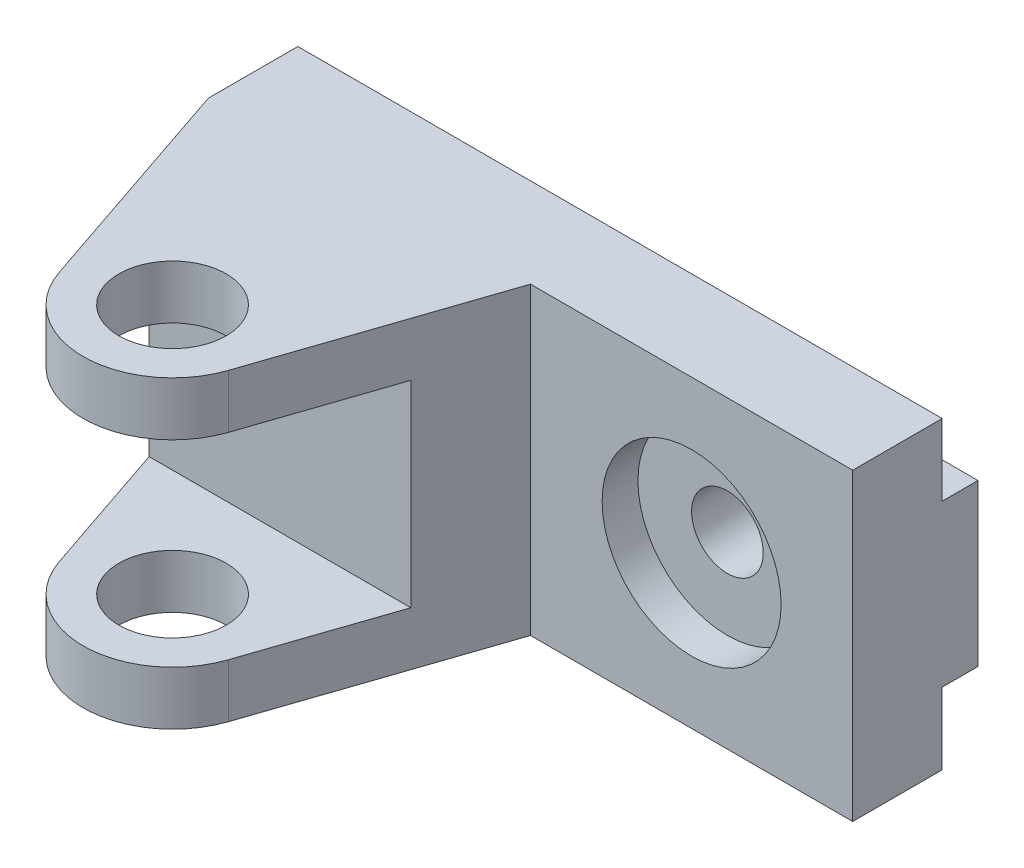
ISO-10303-21;
HEADER;
FILE_DESCRIPTION(('STEP AP214'),'2;1');
FILE_NAME('part.step','',(''),(''),'','','');
FILE_SCHEMA(('AUTOMOTIVE_DESIGN { 1 0 10303 214 1 1 1 1 }'));
ENDSEC;
DATA;
#1=APPLICATION_CONTEXT('core data for automotive mechanical design processes');
#2=APPLICATION_PROTOCOL_DEFINITION('international standard','automotive_design',2000,#1);
#3=PRODUCT_CONTEXT('',#1,'mechanical');
#4=PRODUCT('Part','Part','',(#3));
#5=PRODUCT_RELATED_PRODUCT_CATEGORY('part','',(#4));
#6=PRODUCT_DEFINITION_FORMATION('','',#4);
#7=PRODUCT_DEFINITION_CONTEXT('part definition',#1,'design');
#8=PRODUCT_DEFINITION('design','',#6,#7);
#9=PRODUCT_DEFINITION_SHAPE('','',#8);
#10=(LENGTH_UNIT() NAMED_UNIT(*) SI_UNIT(.MILLI.,.METRE.));
#11=(NAMED_UNIT(*) PLANE_ANGLE_UNIT() SI_UNIT($,.RADIAN.));
#12=(NAMED_UNIT(*) SI_UNIT($,.STERADIAN.) SOLID_ANGLE_UNIT());
#13=UNCERTAINTY_MEASURE_WITH_UNIT(LENGTH_MEASURE(1.E-05),#10,'distance_accuracy_value','');
#14=(GEOMETRIC_REPRESENTATION_CONTEXT(3) GLOBAL_UNCERTAINTY_ASSIGNED_CONTEXT((#13)) GLOBAL_UNIT_ASSIGNED_CONTEXT((#10,
#11,#12)) REPRESENTATION_CONTEXT('',''));
#15=CARTESIAN_POINT('',(0.,0.,0.));
#16=DIRECTION('',(0.,0.,1.));
#17=DIRECTION('',(1.,0.,0.));
#18=AXIS2_PLACEMENT_3D('',#15,#16,#17);
#19=CARTESIAN_POINT('',(0.,0.,25.));
#20=DIRECTION('',(0.,0.,-1.));
#21=DIRECTION('',(-1.,0.,0.));
#22=AXIS2_PLACEMENT_3D('',#19,#20,#21);
#23=PLANE('',#22);
#24=CARTESIAN_POINT('',(45.,0.,25.));
#25=DIRECTION('',(0.,0.,1.));
#26=DIRECTION('',(1.,0.,0.));
#27=AXIS2_PLACEMENT_3D('',#24,#25,#26);
#28=CIRCLE('',#27,25.);
#29=CARTESIAN_POINT('',(70.,0.,25.));
#30=VERTEX_POINT('',#29);
#31=EDGE_CURVE('E242',#30,#30,#28,.T.);
#32=ORIENTED_EDGE('',*,*,#31,.F.);
#33=EDGE_LOOP('',(#32));
#34=FACE_BOUND('',#33,.T.);
#35=DIRECTION('',(-1.,0.,0.));
#36=VECTOR('',#35,1.);
#37=CARTESIAN_POINT('',(-90.,42.5,25.));
#38=LINE('',#37,#36);
#39=CARTESIAN_POINT('',(90.,42.5,25.));
#40=VERTEX_POINT('',#39);
#41=CARTESIAN_POINT('',(0.,42.5,25.));
#42=VERTEX_POINT('',#41);
#43=EDGE_CURVE('E251',#40,#42,#38,.T.);
#44=ORIENTED_EDGE('',*,*,#43,.T.);
#45=DIRECTION('',(0.,-1.,0.));
#46=VECTOR('',#45,1.);
#47=CARTESIAN_POINT('',(0.,-27.5,25.));
#48=LINE('',#47,#46);
#49=CARTESIAN_POINT('',(0.,-42.5,25.));
#50=VERTEX_POINT('',#49);
#51=EDGE_CURVE('E62',#42,#50,#48,.T.);
#52=ORIENTED_EDGE('',*,*,#51,.T.);
#53=DIRECTION('',(1.,0.,0.));
#54=VECTOR('',#53,1.);
#55=CARTESIAN_POINT('',(-90.,-42.5,25.));
#56=LINE('',#55,#54);
#57=CARTESIAN_POINT('',(90.,-42.5,25.));
#58=VERTEX_POINT('',#57);
#59=EDGE_CURVE('E256',#50,#58,#56,.T.);
#60=ORIENTED_EDGE('',*,*,#59,.T.);
#61=DIRECTION('',(0.,1.,0.));
#62=VECTOR('',#61,1.);
#63=CARTESIAN_POINT('',(90.,-42.5,25.));
#64=LINE('',#63,#62);
#65=EDGE_CURVE('E252',#58,#40,#64,.T.);
#66=ORIENTED_EDGE('',*,*,#65,.T.);
#67=EDGE_LOOP('',(#44,#52,#60,#66));
#68=FACE_BOUND('',#67,.T.);
#69=ADVANCED_FACE('F39',(#34,#68),#23,.F.);
#70=CARTESIAN_POINT('',(0.,0.,0.));
#71=DIRECTION('',(0.,0.,-1.));
#72=DIRECTION('',(-1.,0.,0.));
#73=AXIS2_PLACEMENT_3D('',#70,#71,#72);
#74=PLANE('',#73);
#75=DIRECTION('',(0.,1.,0.));
#76=VECTOR('',#75,1.);
#77=CARTESIAN_POINT('',(90.,-42.5,0.));
#78=LINE('',#77,#76);
#79=CARTESIAN_POINT('',(90.,22.5,0.));
#80=VERTEX_POINT('',#79);
#81=CARTESIAN_POINT('',(90.,42.5,0.));
#82=VERTEX_POINT('',#81);
#83=EDGE_CURVE('E247',#80,#82,#78,.T.);
#84=ORIENTED_EDGE('',*,*,#83,.F.);
#85=DIRECTION('',(-1.,0.,0.));
#86=VECTOR('',#85,1.);
#87=CARTESIAN_POINT('',(90.,22.5,0.));
#88=LINE('',#87,#86);
#89=CARTESIAN_POINT('',(-90.,22.5,0.));
#90=VERTEX_POINT('',#89);
#91=EDGE_CURVE('E221',#80,#90,#88,.T.);
#92=ORIENTED_EDGE('',*,*,#91,.T.);
#93=DIRECTION('',(0.,-1.,0.));
#94=VECTOR('',#93,1.);
#95=CARTESIAN_POINT('',(-90.,-42.5,0.));
#96=LINE('',#95,#94);
#97=CARTESIAN_POINT('',(-90.,42.5,0.));
#98=VERTEX_POINT('',#97);
#99=EDGE_CURVE('E267',#98,#90,#96,.T.);
#100=ORIENTED_EDGE('',*,*,#99,.F.);
#101=DIRECTION('',(-1.,0.,0.));
#102=VECTOR('',#101,1.);
#103=CARTESIAN_POINT('',(-90.,42.5,0.));
#104=LINE('',#103,#102);
#105=EDGE_CURVE('E263',#82,#98,#104,.T.);
#106=ORIENTED_EDGE('',*,*,#105,.F.);
#107=EDGE_LOOP('',(#84,#92,#100,#106));
#108=FACE_BOUND('',#107,.T.);
#109=ADVANCED_FACE('F316',(#108),#74,.T.);
#110=CARTESIAN_POINT('',(90.,-42.5,25.));
#111=DIRECTION('',(-1.,0.,0.));
#112=DIRECTION('',(0.,0.,1.));
#113=AXIS2_PLACEMENT_3D('',#110,#111,#112);
#114=PLANE('',#113);
#115=CARTESIAN_POINT('',(90.,-42.5,0.));
#116=VERTEX_POINT('',#115);
#117=CARTESIAN_POINT('',(90.,-22.5,0.));
#118=VERTEX_POINT('',#117);
#119=EDGE_CURVE('E264',#116,#118,#78,.T.);
#120=ORIENTED_EDGE('',*,*,#119,.T.);
#121=DIRECTION('',(0.,0.,1.));
#122=VECTOR('',#121,1.);
#123=CARTESIAN_POINT('',(90.,-22.5,0.));
#124=LINE('',#123,#122);
#125=CARTESIAN_POINT('',(90.,-22.5,-9.99999999999999));
#126=VERTEX_POINT('',#125);
#127=EDGE_CURVE('E222',#126,#118,#124,.T.);
#128=ORIENTED_EDGE('',*,*,#127,.F.);
#129=DIRECTION('',(0.,-1.,0.));
#130=VECTOR('',#129,1.);
#131=CARTESIAN_POINT('',(90.,22.5,-9.99999999999999));
#132=LINE('',#131,#130);
#133=CARTESIAN_POINT('',(90.,22.5,-9.99999999999999));
#134=VERTEX_POINT('',#133);
#135=EDGE_CURVE('E216',#134,#126,#132,.T.);
#136=ORIENTED_EDGE('',*,*,#135,.F.);
#137=DIRECTION('',(0.,0.,-1.));
#138=VECTOR('',#137,1.);
#139=CARTESIAN_POINT('',(90.,22.5,0.));
#140=LINE('',#139,#138);
#141=EDGE_CURVE('E217',#80,#134,#140,.T.);
#142=ORIENTED_EDGE('',*,*,#141,.F.);
#143=ORIENTED_EDGE('',*,*,#83,.T.);
#144=DIRECTION('',(0.,0.,-1.));
#145=VECTOR('',#144,1.);
#146=CARTESIAN_POINT('',(90.,42.5,25.));
#147=LINE('',#146,#145);
#148=EDGE_CURVE('E160',#40,#82,#147,.T.);
#149=ORIENTED_EDGE('',*,*,#148,.F.);
#150=ORIENTED_EDGE('',*,*,#65,.F.);
#151=DIRECTION('',(0.,0.,-1.));
#152=VECTOR('',#151,1.);
#153=CARTESIAN_POINT('',(90.,-42.5,25.));
#154=LINE('',#153,#152);
#155=EDGE_CURVE('E262',#58,#116,#154,.T.);
#156=ORIENTED_EDGE('',*,*,#155,.T.);
#157=EDGE_LOOP('',(#120,#128,#136,#142,#143,#149,#150,#156));
#158=FACE_BOUND('',#157,.T.);
#159=ADVANCED_FACE('F41',(#158),#114,.F.);
#160=CARTESIAN_POINT('',(-90.,42.5,25.));
#161=DIRECTION('',(0.,-1.,0.));
#162=DIRECTION('',(0.,0.,-1.));
#163=AXIS2_PLACEMENT_3D('',#160,#161,#162);
#164=PLANE('',#163);
#165=ORIENTED_EDGE('',*,*,#105,.T.);
#166=DIRECTION('',(0.,0.,-1.));
#167=VECTOR('',#166,1.);
#168=CARTESIAN_POINT('',(-90.,42.5,25.));
#169=LINE('',#168,#167);
#170=CARTESIAN_POINT('',(-90.,42.5,25.));
#171=VERTEX_POINT('',#170);
#172=EDGE_CURVE('E280',#171,#98,#169,.T.);
#173=ORIENTED_EDGE('',*,*,#172,.F.);
#174=DIRECTION('',(0.320481248816092,0.,0.947254859664113));
#175=VECTOR('',#174,1.);
#176=CARTESIAN_POINT('',(-90.,42.5,25.));
#177=LINE('',#176,#175);
#178=CARTESIAN_POINT('',(-68.6813714916028,42.5,88.0120312204023));
#179=VERTEX_POINT('',#178);
#180=EDGE_CURVE('E178',#171,#179,#177,.T.);
#181=ORIENTED_EDGE('',*,*,#180,.T.);
#182=CARTESIAN_POINT('',(-45.,42.5,80.));
#183=DIRECTION('',(0.,1.,0.));
#184=DIRECTION('',(0.,0.,1.));
#185=AXIS2_PLACEMENT_3D('',#182,#183,#184);
#186=CIRCLE('',#185,25.);
#187=CARTESIAN_POINT('',(-21.3186285083972,42.5,88.0120312204023));
#188=VERTEX_POINT('',#187);
#189=EDGE_CURVE('E167',#179,#188,#186,.T.);
#190=ORIENTED_EDGE('',*,*,#189,.T.);
#191=DIRECTION('',(0.320481248816092,0.,-0.947254859664113));
#192=VECTOR('',#191,1.);
#193=CARTESIAN_POINT('',(0.,42.5,25.));
#194=LINE('',#193,#192);
#195=EDGE_CURVE('E164',#188,#42,#194,.T.);
#196=ORIENTED_EDGE('',*,*,#195,.T.);
#197=ORIENTED_EDGE('',*,*,#43,.F.);
#198=ORIENTED_EDGE('',*,*,#148,.T.);
#199=EDGE_LOOP('',(#165,#173,#181,#190,#196,#197,#198));
#200=FACE_BOUND('',#199,.T.);
#201=CARTESIAN_POINT('',(-45.,42.5,80.));
#202=DIRECTION('',(0.,1.,0.));
#203=DIRECTION('',(0.,0.,1.));
#204=AXIS2_PLACEMENT_3D('',#201,#202,#203);
#205=CIRCLE('',#204,15.);
#206=CARTESIAN_POINT('',(-45.,42.5,95.));
#207=VERTEX_POINT('',#206);
#208=EDGE_CURVE('E173',#207,#207,#205,.T.);
#209=ORIENTED_EDGE('',*,*,#208,.F.);
#210=EDGE_LOOP('',(#209));
#211=FACE_BOUND('',#210,.T.);
#212=ADVANCED_FACE('F310',(#200,#211),#164,.F.);
#213=CARTESIAN_POINT('',(-90.,-42.5,25.));
#214=DIRECTION('',(1.,0.,0.));
#215=DIRECTION('',(0.,0.,-1.));
#216=AXIS2_PLACEMENT_3D('',#213,#214,#215);
#217=PLANE('',#216);
#218=DIRECTION('',(0.,0.,-1.));
#219=VECTOR('',#218,1.);
#220=CARTESIAN_POINT('',(-90.,-42.5,25.));
#221=LINE('',#220,#219);
#222=CARTESIAN_POINT('',(-90.,-42.5,25.));
#223=VERTEX_POINT('',#222);
#224=CARTESIAN_POINT('',(-90.,-42.5,0.));
#225=VERTEX_POINT('',#224);
#226=EDGE_CURVE('E274',#223,#225,#221,.T.);
#227=ORIENTED_EDGE('',*,*,#226,.F.);
#228=DIRECTION('',(0.,-1.,0.));
#229=VECTOR('',#228,1.);
#230=CARTESIAN_POINT('',(-90.,-42.5,25.));
#231=LINE('',#230,#229);
#232=EDGE_CURVE('E260',#171,#223,#231,.T.);
#233=ORIENTED_EDGE('',*,*,#232,.F.);
#234=ORIENTED_EDGE('',*,*,#172,.T.);
#235=ORIENTED_EDGE('',*,*,#99,.T.);
#236=DIRECTION('',(0.,0.,-1.));
#237=VECTOR('',#236,1.);
#238=CARTESIAN_POINT('',(-90.,22.5,0.));
#239=LINE('',#238,#237);
#240=CARTESIAN_POINT('',(-90.,22.5,-9.99999999999999));
#241=VERTEX_POINT('',#240);
#242=EDGE_CURVE('E213',#90,#241,#239,.T.);
#243=ORIENTED_EDGE('',*,*,#242,.T.);
#244=DIRECTION('',(0.,-1.,0.));
#245=VECTOR('',#244,1.);
#246=CARTESIAN_POINT('',(-90.,22.5,-9.99999999999999));
#247=LINE('',#246,#245);
#248=CARTESIAN_POINT('',(-90.,-22.5,-9.99999999999999));
#249=VERTEX_POINT('',#248);
#250=EDGE_CURVE('E226',#241,#249,#247,.T.);
#251=ORIENTED_EDGE('',*,*,#250,.T.);
#252=DIRECTION('',(0.,0.,1.));
#253=VECTOR('',#252,1.);
#254=CARTESIAN_POINT('',(-90.,-22.5,0.));
#255=LINE('',#254,#253);
#256=CARTESIAN_POINT('',(-90.,-22.5,0.));
#257=VERTEX_POINT('',#256);
#258=EDGE_CURVE('E218',#249,#257,#255,.T.);
#259=ORIENTED_EDGE('',*,*,#258,.T.);
#260=EDGE_CURVE('E269',#257,#225,#96,.T.);
#261=ORIENTED_EDGE('',*,*,#260,.T.);
#262=EDGE_LOOP('',(#227,#233,#234,#235,#243,#251,#259,#261));
#263=FACE_BOUND('',#262,.T.);
#264=ADVANCED_FACE('F320',(#263),#217,.F.);
#265=CARTESIAN_POINT('',(-90.,-42.5,25.));
#266=DIRECTION('',(0.,1.,0.));
#267=DIRECTION('',(0.,0.,1.));
#268=AXIS2_PLACEMENT_3D('',#265,#266,#267);
#269=PLANE('',#268);
#270=DIRECTION('',(1.,0.,0.));
#271=VECTOR('',#270,1.);
#272=CARTESIAN_POINT('',(-90.,-42.5,0.));
#273=LINE('',#272,#271);
#274=EDGE_CURVE('E253',#225,#116,#273,.T.);
#275=ORIENTED_EDGE('',*,*,#274,.T.);
#276=ORIENTED_EDGE('',*,*,#155,.F.);
#277=ORIENTED_EDGE('',*,*,#59,.F.);
#278=DIRECTION('',(-0.320481248816092,0.,0.947254859664113));
#279=VECTOR('',#278,1.);
#280=CARTESIAN_POINT('',(-21.3186285083972,-42.5,88.0120312204023));
#281=LINE('',#280,#279);
#282=CARTESIAN_POINT('',(-21.3186285083972,-42.5,88.0120312204023));
#283=VERTEX_POINT('',#282);
#284=EDGE_CURVE('E188',#50,#283,#281,.T.);
#285=ORIENTED_EDGE('',*,*,#284,.T.);
#286=CARTESIAN_POINT('',(-45.,-42.5,80.));
#287=DIRECTION('',(0.,-1.,0.));
#288=DIRECTION('',(0.,0.,-1.));
#289=AXIS2_PLACEMENT_3D('',#286,#287,#288);
#290=CIRCLE('',#289,25.);
#291=CARTESIAN_POINT('',(-68.6813714916028,-42.5,88.0120312204023));
#292=VERTEX_POINT('',#291);
#293=EDGE_CURVE('E203',#283,#292,#290,.T.);
#294=ORIENTED_EDGE('',*,*,#293,.T.);
#295=DIRECTION('',(-0.320481248816092,0.,-0.947254859664113));
#296=VECTOR('',#295,1.);
#297=CARTESIAN_POINT('',(-68.6813714916028,-42.5,88.0120312204023));
#298=LINE('',#297,#296);
#299=EDGE_CURVE('E197',#292,#223,#298,.T.);
#300=ORIENTED_EDGE('',*,*,#299,.T.);
#301=ORIENTED_EDGE('',*,*,#226,.T.);
#302=EDGE_LOOP('',(#275,#276,#277,#285,#294,#300,#301));
#303=FACE_BOUND('',#302,.T.);
#304=CARTESIAN_POINT('',(-45.,-42.5,80.));
#305=DIRECTION('',(0.,-1.,0.));
#306=DIRECTION('',(0.,0.,-1.));
#307=AXIS2_PLACEMENT_3D('',#304,#305,#306);
#308=CIRCLE('',#307,15.);
#309=CARTESIAN_POINT('',(-45.,-42.5,65.));
#310=VERTEX_POINT('',#309);
#311=EDGE_CURVE('E184',#310,#310,#308,.T.);
#312=ORIENTED_EDGE('',*,*,#311,.F.);
#313=EDGE_LOOP('',(#312));
#314=FACE_BOUND('',#313,.T.);
#315=ADVANCED_FACE('F298',(#303,#314),#269,.F.);
#316=DIRECTION('',(-1.,0.,0.));
#317=VECTOR('',#316,1.);
#318=CARTESIAN_POINT('',(90.,-22.5,0.));
#319=LINE('',#318,#317);
#320=EDGE_CURVE('E231',#118,#257,#319,.T.);
#321=ORIENTED_EDGE('',*,*,#320,.F.);
#322=ORIENTED_EDGE('',*,*,#119,.F.);
#323=ORIENTED_EDGE('',*,*,#274,.F.);
#324=ORIENTED_EDGE('',*,*,#260,.F.);
#325=EDGE_LOOP('',(#321,#322,#323,#324));
#326=FACE_BOUND('',#325,.T.);
#327=ADVANCED_FACE('F332',(#326),#74,.T.);
#328=CARTESIAN_POINT('',(45.,0.,15.));
#329=DIRECTION('',(0.,0.,1.));
#330=DIRECTION('',(1.,0.,0.));
#331=AXIS2_PLACEMENT_3D('',#328,#329,#330);
#332=CYLINDRICAL_SURFACE('',#331,25.);
#333=CARTESIAN_POINT('',(45.,0.,15.));
#334=DIRECTION('',(0.,0.,1.));
#335=DIRECTION('',(1.,0.,0.));
#336=AXIS2_PLACEMENT_3D('',#333,#334,#335);
#337=CIRCLE('',#336,25.);
#338=CARTESIAN_POINT('',(70.,0.,15.));
#339=VERTEX_POINT('',#338);
#340=EDGE_CURVE('E244',#339,#339,#337,.T.);
#341=ORIENTED_EDGE('',*,*,#340,.F.);
#342=EDGE_LOOP('',(#341));
#343=FACE_BOUND('',#342,.T.);
#344=ORIENTED_EDGE('',*,*,#31,.T.);
#345=EDGE_LOOP('',(#344));
#346=FACE_BOUND('',#345,.T.);
#347=ADVANCED_FACE('F331',(#343,#346),#332,.F.);
#348=CARTESIAN_POINT('',(45.,0.,15.));
#349=DIRECTION('',(0.,0.,1.));
#350=DIRECTION('',(1.,0.,0.));
#351=AXIS2_PLACEMENT_3D('',#348,#349,#350);
#352=PLANE('',#351);
#353=CARTESIAN_POINT('',(45.,0.,15.));
#354=DIRECTION('',(0.,0.,1.));
#355=DIRECTION('',(1.,0.,0.));
#356=AXIS2_PLACEMENT_3D('',#353,#354,#355);
#357=CIRCLE('',#356,10.);
#358=CARTESIAN_POINT('',(55.,0.,15.));
#359=VERTEX_POINT('',#358);
#360=EDGE_CURVE('E232',#359,#359,#357,.T.);
#361=ORIENTED_EDGE('',*,*,#360,.F.);
#362=EDGE_LOOP('',(#361));
#363=FACE_BOUND('',#362,.T.);
#364=ORIENTED_EDGE('',*,*,#340,.T.);
#365=EDGE_LOOP('',(#364));
#366=FACE_BOUND('',#365,.T.);
#367=ADVANCED_FACE('F345',(#363,#366),#352,.T.);
#368=CARTESIAN_POINT('',(45.,0.,-5.));
#369=DIRECTION('',(0.,0.,1.));
#370=DIRECTION('',(1.,0.,0.));
#371=AXIS2_PLACEMENT_3D('',#368,#369,#370);
#372=CYLINDRICAL_SURFACE('',#371,10.);
#373=ORIENTED_EDGE('',*,*,#360,.T.);
#374=EDGE_LOOP('',(#373));
#375=FACE_BOUND('',#374,.T.);
#376=CARTESIAN_POINT('',(45.,0.,-9.99999999999999));
#377=DIRECTION('',(0.,0.,1.));
#378=DIRECTION('',(1.,0.,0.));
#379=AXIS2_PLACEMENT_3D('',#376,#377,#378);
#380=CIRCLE('',#379,10.);
#381=CARTESIAN_POINT('',(55.,0.,-9.99999999999999));
#382=VERTEX_POINT('',#381);
#383=EDGE_CURVE('E206',#382,#382,#380,.T.);
#384=ORIENTED_EDGE('',*,*,#383,.F.);
#385=EDGE_LOOP('',(#384));
#386=FACE_BOUND('',#385,.T.);
#387=ADVANCED_FACE('F356',(#375,#386),#372,.F.);
#388=CARTESIAN_POINT('',(90.,22.5,0.));
#389=DIRECTION('',(0.,1.,0.));
#390=DIRECTION('',(0.,0.,1.));
#391=AXIS2_PLACEMENT_3D('',#388,#389,#390);
#392=PLANE('',#391);
#393=ORIENTED_EDGE('',*,*,#242,.F.);
#394=ORIENTED_EDGE('',*,*,#91,.F.);
#395=ORIENTED_EDGE('',*,*,#141,.T.);
#396=DIRECTION('',(-1.,0.,0.));
#397=VECTOR('',#396,1.);
#398=CARTESIAN_POINT('',(90.,22.5,-9.99999999999999));
#399=LINE('',#398,#397);
#400=EDGE_CURVE('E238',#134,#241,#399,.T.);
#401=ORIENTED_EDGE('',*,*,#400,.T.);
#402=EDGE_LOOP('',(#393,#394,#395,#401));
#403=FACE_BOUND('',#402,.T.);
#404=ADVANCED_FACE('F322',(#403),#392,.T.);
#405=CARTESIAN_POINT('',(90.,22.5,-9.99999999999999));
#406=DIRECTION('',(0.,0.,-1.));
#407=DIRECTION('',(0.,1.,0.));
#408=AXIS2_PLACEMENT_3D('',#405,#406,#407);
#409=PLANE('',#408);
#410=ORIENTED_EDGE('',*,*,#383,.T.);
#411=EDGE_LOOP('',(#410));
#412=FACE_BOUND('',#411,.T.);
#413=ORIENTED_EDGE('',*,*,#250,.F.);
#414=ORIENTED_EDGE('',*,*,#400,.F.);
#415=ORIENTED_EDGE('',*,*,#135,.T.);
#416=DIRECTION('',(-1.,0.,0.));
#417=VECTOR('',#416,1.);
#418=CARTESIAN_POINT('',(90.,-22.5,-9.99999999999999));
#419=LINE('',#418,#417);
#420=EDGE_CURVE('E236',#126,#249,#419,.T.);
#421=ORIENTED_EDGE('',*,*,#420,.T.);
#422=EDGE_LOOP('',(#413,#414,#415,#421));
#423=FACE_BOUND('',#422,.T.);
#424=ADVANCED_FACE('F327',(#412,#423),#409,.T.);
#425=CARTESIAN_POINT('',(90.,-22.5,0.));
#426=DIRECTION('',(0.,-1.,0.));
#427=DIRECTION('',(0.,0.,-1.));
#428=AXIS2_PLACEMENT_3D('',#425,#426,#427);
#429=PLANE('',#428);
#430=ORIENTED_EDGE('',*,*,#258,.F.);
#431=ORIENTED_EDGE('',*,*,#420,.F.);
#432=ORIENTED_EDGE('',*,*,#127,.T.);
#433=ORIENTED_EDGE('',*,*,#320,.T.);
#434=EDGE_LOOP('',(#430,#431,#432,#433));
#435=FACE_BOUND('',#434,.T.);
#436=ADVANCED_FACE('F328',(#435),#429,.T.);
#437=CARTESIAN_POINT('',(-68.6813714916028,-27.5,88.0120312204023));
#438=DIRECTION('',(-0.947254859664113,0.,0.320481248816092));
#439=DIRECTION('',(0.320481248816092,0.,0.947254859664113));
#440=AXIS2_PLACEMENT_3D('',#437,#438,#439);
#441=PLANE('',#440);
#442=ORIENTED_EDGE('',*,*,#299,.F.);
#443=DIRECTION('',(0.,-1.,0.));
#444=VECTOR('',#443,1.);
#445=CARTESIAN_POINT('',(-68.6813714916028,-27.5,88.0120312204023));
#446=LINE('',#445,#444);
#447=CARTESIAN_POINT('',(-68.6813714916028,-27.5,88.0120312204023));
#448=VERTEX_POINT('',#447);
#449=EDGE_CURVE('E207',#448,#292,#446,.T.);
#450=ORIENTED_EDGE('',*,*,#449,.F.);
#451=DIRECTION('',(-0.320481248816092,0.,-0.947254859664113));
#452=VECTOR('',#451,1.);
#453=CARTESIAN_POINT('',(-68.6813714916028,-27.5,88.0120312204023));
#454=LINE('',#453,#452);
#455=CARTESIAN_POINT('',(-81.5418420516277,-27.5,50.));
#456=VERTEX_POINT('',#455);
#457=EDGE_CURVE('E154',#448,#456,#454,.T.);
#458=ORIENTED_EDGE('',*,*,#457,.T.);
#459=DIRECTION('',(0.,1.,0.));
#460=VECTOR('',#459,1.);
#461=CARTESIAN_POINT('',(-81.5418420516277,0.,50.));
#462=LINE('',#461,#460);
#463=CARTESIAN_POINT('',(-81.5418420516277,27.5,50.));
#464=VERTEX_POINT('',#463);
#465=EDGE_CURVE('E11',#456,#464,#462,.T.);
#466=ORIENTED_EDGE('',*,*,#465,.T.);
#467=DIRECTION('',(0.320481248816092,0.,0.947254859664113));
#468=VECTOR('',#467,1.);
#469=CARTESIAN_POINT('',(-90.,27.5,25.));
#470=LINE('',#469,#468);
#471=CARTESIAN_POINT('',(-68.6813714916028,27.5,88.0120312204023));
#472=VERTEX_POINT('',#471);
#473=EDGE_CURVE('E146',#464,#472,#470,.T.);
#474=ORIENTED_EDGE('',*,*,#473,.T.);
#475=DIRECTION('',(0.,1.,0.));
#476=VECTOR('',#475,1.);
#477=CARTESIAN_POINT('',(-68.6813714916028,27.5,88.0120312204023));
#478=LINE('',#477,#476);
#479=EDGE_CURVE('E180',#472,#179,#478,.T.);
#480=ORIENTED_EDGE('',*,*,#479,.T.);
#481=ORIENTED_EDGE('',*,*,#180,.F.);
#482=ORIENTED_EDGE('',*,*,#232,.T.);
#483=EDGE_LOOP('',(#442,#450,#458,#466,#474,#480,#481,#482));
#484=FACE_BOUND('',#483,.T.);
#485=ADVANCED_FACE('F147',(#484),#441,.T.);
#486=CARTESIAN_POINT('',(-45.,-27.5,80.));
#487=DIRECTION('',(0.,-1.,0.));
#488=DIRECTION('',(0.,0.,-1.));
#489=AXIS2_PLACEMENT_3D('',#486,#487,#488);
#490=CYLINDRICAL_SURFACE('',#489,25.);
#491=ORIENTED_EDGE('',*,*,#293,.F.);
#492=DIRECTION('',(0.,-1.,0.));
#493=VECTOR('',#492,1.);
#494=CARTESIAN_POINT('',(-21.3186285083972,-27.5,88.0120312204023));
#495=LINE('',#494,#493);
#496=CARTESIAN_POINT('',(-21.3186285083972,-27.5,88.0120312204023));
#497=VERTEX_POINT('',#496);
#498=EDGE_CURVE('E209',#497,#283,#495,.T.);
#499=ORIENTED_EDGE('',*,*,#498,.F.);
#500=CARTESIAN_POINT('',(-45.,-27.5,80.));
#501=DIRECTION('',(0.,-1.,0.));
#502=DIRECTION('',(0.,0.,-1.));
#503=AXIS2_PLACEMENT_3D('',#500,#501,#502);
#504=CIRCLE('',#503,25.);
#505=EDGE_CURVE('E193',#497,#448,#504,.T.);
#506=ORIENTED_EDGE('',*,*,#505,.T.);
#507=ORIENTED_EDGE('',*,*,#449,.T.);
#508=EDGE_LOOP('',(#491,#499,#506,#507));
#509=FACE_BOUND('',#508,.T.);
#510=ADVANCED_FACE('F293',(#509),#490,.T.);
#511=CARTESIAN_POINT('',(-21.3186285083972,-27.5,88.0120312204023));
#512=DIRECTION('',(0.947254859664113,0.,0.320481248816092));
#513=DIRECTION('',(0.320481248816092,0.,-0.947254859664113));
#514=AXIS2_PLACEMENT_3D('',#511,#512,#513);
#515=PLANE('',#514);
#516=ORIENTED_EDGE('',*,*,#498,.T.);
#517=ORIENTED_EDGE('',*,*,#284,.F.);
#518=ORIENTED_EDGE('',*,*,#51,.F.);
#519=ORIENTED_EDGE('',*,*,#195,.F.);
#520=DIRECTION('',(0.,1.,0.));
#521=VECTOR('',#520,1.);
#522=CARTESIAN_POINT('',(-21.3186285083972,27.5,88.0120312204023));
#523=LINE('',#522,#521);
#524=CARTESIAN_POINT('',(-21.3186285083972,27.5,88.0120312204023));
#525=VERTEX_POINT('',#524);
#526=EDGE_CURVE('E182',#525,#188,#523,.T.);
#527=ORIENTED_EDGE('',*,*,#526,.F.);
#528=DIRECTION('',(0.320481248816092,0.,-0.947254859664113));
#529=VECTOR('',#528,1.);
#530=CARTESIAN_POINT('',(0.,27.5,25.));
#531=LINE('',#530,#529);
#532=CARTESIAN_POINT('',(-8.4581579483723,27.5,50.));
#533=VERTEX_POINT('',#532);
#534=EDGE_CURVE('E170',#525,#533,#531,.T.);
#535=ORIENTED_EDGE('',*,*,#534,.T.);
#536=DIRECTION('',(0.,-1.,0.));
#537=VECTOR('',#536,1.);
#538=CARTESIAN_POINT('',(-8.4581579483723,0.,50.));
#539=LINE('',#538,#537);
#540=CARTESIAN_POINT('',(-8.4581579483723,-27.5,50.));
#541=VERTEX_POINT('',#540);
#542=EDGE_CURVE('E50',#533,#541,#539,.T.);
#543=ORIENTED_EDGE('',*,*,#542,.T.);
#544=DIRECTION('',(-0.320481248816092,0.,0.947254859664113));
#545=VECTOR('',#544,1.);
#546=CARTESIAN_POINT('',(-21.3186285083972,-27.5,88.0120312204023));
#547=LINE('',#546,#545);
#548=EDGE_CURVE('E194',#541,#497,#547,.T.);
#549=ORIENTED_EDGE('',*,*,#548,.T.);
#550=EDGE_LOOP('',(#516,#517,#518,#519,#527,#535,#543,#549));
#551=FACE_BOUND('',#550,.T.);
#552=ADVANCED_FACE('F282',(#551),#515,.T.);
#553=CARTESIAN_POINT('',(-45.,-27.5,80.));
#554=DIRECTION('',(0.,-1.,0.));
#555=DIRECTION('',(0.,0.,-1.));
#556=AXIS2_PLACEMENT_3D('',#553,#554,#555);
#557=PLANE('',#556);
#558=CARTESIAN_POINT('',(-45.,-27.5,80.));
#559=DIRECTION('',(0.,-1.,0.));
#560=DIRECTION('',(0.,0.,-1.));
#561=AXIS2_PLACEMENT_3D('',#558,#559,#560);
#562=CIRCLE('',#561,15.);
#563=CARTESIAN_POINT('',(-45.,-27.5,65.));
#564=VERTEX_POINT('',#563);
#565=EDGE_CURVE('E190',#564,#564,#562,.T.);
#566=ORIENTED_EDGE('',*,*,#565,.T.);
#567=EDGE_LOOP('',(#566));
#568=FACE_BOUND('',#567,.T.);
#569=ORIENTED_EDGE('',*,*,#548,.F.);
#570=DIRECTION('',(1.,0.,0.));
#571=VECTOR('',#570,1.);
#572=CARTESIAN_POINT('',(-90.,-27.5,50.));
#573=LINE('',#572,#571);
#574=EDGE_CURVE('E281',#456,#541,#573,.T.);
#575=ORIENTED_EDGE('',*,*,#574,.F.);
#576=ORIENTED_EDGE('',*,*,#457,.F.);
#577=ORIENTED_EDGE('',*,*,#505,.F.);
#578=EDGE_LOOP('',(#569,#575,#576,#577));
#579=FACE_BOUND('',#578,.T.);
#580=ADVANCED_FACE('F287',(#568,#579),#557,.F.);
#581=CARTESIAN_POINT('',(-45.,-27.5,80.));
#582=DIRECTION('',(0.,-1.,0.));
#583=DIRECTION('',(0.,0.,-1.));
#584=AXIS2_PLACEMENT_3D('',#581,#582,#583);
#585=CYLINDRICAL_SURFACE('',#584,15.);
#586=ORIENTED_EDGE('',*,*,#565,.F.);
#587=EDGE_LOOP('',(#586));
#588=FACE_BOUND('',#587,.T.);
#589=ORIENTED_EDGE('',*,*,#311,.T.);
#590=EDGE_LOOP('',(#589));
#591=FACE_BOUND('',#590,.T.);
#592=ADVANCED_FACE('F380',(#588,#591),#585,.F.);
#593=CARTESIAN_POINT('',(-45.,27.5,80.));
#594=DIRECTION('',(0.,1.,0.));
#595=DIRECTION('',(0.,0.,1.));
#596=AXIS2_PLACEMENT_3D('',#593,#594,#595);
#597=CYLINDRICAL_SURFACE('',#596,25.);
#598=ORIENTED_EDGE('',*,*,#189,.F.);
#599=ORIENTED_EDGE('',*,*,#479,.F.);
#600=CARTESIAN_POINT('',(-45.,27.5,80.));
#601=DIRECTION('',(0.,1.,0.));
#602=DIRECTION('',(0.,0.,1.));
#603=AXIS2_PLACEMENT_3D('',#600,#601,#602);
#604=CIRCLE('',#603,25.);
#605=EDGE_CURVE('E165',#472,#525,#604,.T.);
#606=ORIENTED_EDGE('',*,*,#605,.T.);
#607=ORIENTED_EDGE('',*,*,#526,.T.);
#608=EDGE_LOOP('',(#598,#599,#606,#607));
#609=FACE_BOUND('',#608,.T.);
#610=ADVANCED_FACE('F315',(#609),#597,.T.);
#611=CARTESIAN_POINT('',(-45.,27.5,80.));
#612=DIRECTION('',(0.,1.,0.));
#613=DIRECTION('',(0.,0.,1.));
#614=AXIS2_PLACEMENT_3D('',#611,#612,#613);
#615=PLANE('',#614);
#616=CARTESIAN_POINT('',(-45.,27.5,80.));
#617=DIRECTION('',(0.,1.,0.));
#618=DIRECTION('',(0.,0.,1.));
#619=AXIS2_PLACEMENT_3D('',#616,#617,#618);
#620=CIRCLE('',#619,15.);
#621=CARTESIAN_POINT('',(-45.,27.5,95.));
#622=VERTEX_POINT('',#621);
#623=EDGE_CURVE('E179',#622,#622,#620,.T.);
#624=ORIENTED_EDGE('',*,*,#623,.T.);
#625=EDGE_LOOP('',(#624));
#626=FACE_BOUND('',#625,.T.);
#627=ORIENTED_EDGE('',*,*,#473,.F.);
#628=DIRECTION('',(1.,0.,0.));
#629=VECTOR('',#628,1.);
#630=CARTESIAN_POINT('',(-45.,27.5,50.));
#631=LINE('',#630,#629);
#632=EDGE_CURVE('E151',#464,#533,#631,.T.);
#633=ORIENTED_EDGE('',*,*,#632,.T.);
#634=ORIENTED_EDGE('',*,*,#534,.F.);
#635=ORIENTED_EDGE('',*,*,#605,.F.);
#636=EDGE_LOOP('',(#627,#633,#634,#635));
#637=FACE_BOUND('',#636,.T.);
#638=ADVANCED_FACE('F162',(#626,#637),#615,.F.);
#639=CARTESIAN_POINT('',(-45.,27.5,80.));
#640=DIRECTION('',(0.,1.,0.));
#641=DIRECTION('',(0.,0.,1.));
#642=AXIS2_PLACEMENT_3D('',#639,#640,#641);
#643=CYLINDRICAL_SURFACE('',#642,15.);
#644=ORIENTED_EDGE('',*,*,#623,.F.);
#645=EDGE_LOOP('',(#644));
#646=FACE_BOUND('',#645,.T.);
#647=ORIENTED_EDGE('',*,*,#208,.T.);
#648=EDGE_LOOP('',(#647));
#649=FACE_BOUND('',#648,.T.);
#650=ADVANCED_FACE('F387',(#646,#649),#643,.F.);
#651=CARTESIAN_POINT('',(0.,0.,50.));
#652=DIRECTION('',(0.,0.,1.));
#653=DIRECTION('',(1.,0.,0.));
#654=AXIS2_PLACEMENT_3D('',#651,#652,#653);
#655=PLANE('',#654);
#656=ORIENTED_EDGE('',*,*,#465,.F.);
#657=ORIENTED_EDGE('',*,*,#574,.T.);
#658=ORIENTED_EDGE('',*,*,#542,.F.);
#659=ORIENTED_EDGE('',*,*,#632,.F.);
#660=EDGE_LOOP('',(#656,#657,#658,#659));
#661=FACE_BOUND('',#660,.T.);
#662=ADVANCED_FACE('F153',(#661),#655,.T.);
#663=CLOSED_SHELL('',(#69,#109,#159,#212,#264,#315,#327,#347,#367,#387,#404,#424,#436,#485,#510,
#552,#580,#592,#610,#638,#650,#662));
#664=MANIFOLD_SOLID_BREP('B2',#663);
#665=ADVANCED_BREP_SHAPE_REPRESENTATION('',(#18,#664),#14);
#666=SHAPE_DEFINITION_REPRESENTATION(#9,#665);
ENDSEC;
END-ISO-10303-21;
